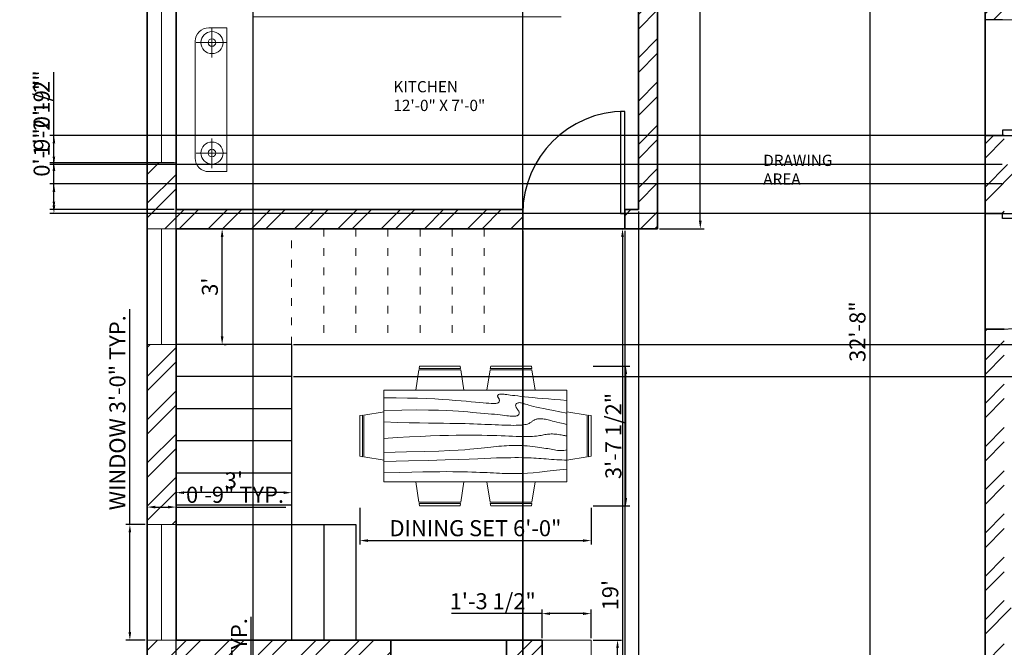
# Model space of a CAD drawing. Units: inches. Extents: x 28986 to 29505, y -162 to 451.
# Tile 3 of 6: x 29011 to 29318, y 32 to 228. Entities that reach past the tile are written whole.
import ezdxf

# ---------------------------------------------------------------- set-up
doc = ezdxf.new("R2010")
doc.units = ezdxf.units.IN
doc.linetypes.add('ACAD_ISO03W100', pattern=[30, 12, -18])
doc.layers.get('Defpoints').update_dxf_attribs({"color": 120})
for name, color, linetype, lineweight, true_color in [('A-ANNO-DIMS', 9, 'Continuous', 18, 0xafd9aa), ('A-FLOR-CASE', 32, 'Continuous', 18, 0xcd6928), ('A-FLOR-STRS', 32, 'Continuous', 25, 0xcd6928), ('A-FLOR-STRS-OVHD', 32, 'ACAD_ISO03W100', 18, 0xcd6928)]:
    doc.layers.add(name, color=color, linetype=linetype, lineweight=lineweight, true_color=true_color)
for name, color, linetype, lineweight in [('A-AREA-IDEN', 6, 'Continuous', 18), ('A-EQPM', 8, 'Continuous', 18), ('A-GLAZ', 4, 'Continuous', 18), ('A-WALL', 7, 'Continuous', 35), ('A-WALL-PATT', 1, 'Continuous', 13), ('DOOR', 2, 'Continuous', 25), ('FURNITURE', 241, 'Continuous', 18)]:
    doc.layers.add(name, color=color, linetype=linetype, lineweight=lineweight)
doc.styles.get("Standard").update_dxf_attribs({"font": 'arial.ttf'})
doc.dimstyles.new('ISO-25', dxfattribs={"dimtxt": 5, "dimasz": 2.5, "dimexe": 1.25, "dimexo": 0.625, "dimtad": 1, "dimdec": 0, "dimlunit": 3, "dimtxsty": 'Standard', "dimcen": 2.5, "dimadec": 0, "dimazin": 0, "dimtfac": 1, "dimtdec": 0, "dimtmove": 0, "dimatfit": 3, "dimfxl": 1, "dimarcsym": 0})

# ---------------------------------------------------------------- blocks, each defined once
blk = doc.blocks.new('*D1')
at = {"layer": 'A-ANNO-DIMS', "color": 0, "lineweight": -2, "transparency": 16777216}
for p, q in [((29075.13, 162.7), (29075.76, 162.7)), ((29074.51, 129.2), (29074.51, 160.2)), ((29075.13, 126.7), (29075.76, 126.7))]:
    blk.add_line(p, q, dxfattribs=at)
at = {"layer": 'A-ANNO-DIMS', "color": 0, "transparency": 16777216}
for points in [[(29074.09, 160.2), (29074.92, 160.2), (29074.51, 162.7)], [(29074.09, 129.2), (29074.92, 129.2), (29074.51, 126.7)]]:
    blk.add_solid(points, dxfattribs=at)
at = {"layer": 'Defpoints', "color": 0, "transparency": 16777216}
for p in [(29074.51, 162.7), (29074.51, 162.7), (29074.51, 126.7)]:
    blk.add_point(p, dxfattribs=at)
at = {"layer": 'A-ANNO-DIMS', "color": 0, "transparency": 16777216, "insert": (29071.33, 144.7), "char_height": 5, "attachment_point": 5, "rotation": 90}
blk.add_mtext("3'", dxfattribs=at)
blk = doc.blocks.new('*D2')
at = {"layer": 'A-ANNO-DIMS', "color": 0, "lineweight": -2, "transparency": 16777216}
for p, q in [((29060.16, 80.07), (29060.16, 79.34)), ((29093.66, 80.59), (29062.66, 80.59)), ((29096.16, 80.07), (29096.16, 79.34))]:
    blk.add_line(p, q, dxfattribs=at)
at = {"layer": 'A-ANNO-DIMS', "color": 0, "transparency": 16777216}
for points in [[(29062.66, 81), (29062.66, 80.17), (29060.16, 80.59)], [(29093.66, 81), (29093.66, 80.17), (29096.16, 80.59)]]:
    blk.add_solid(points, dxfattribs=at)
at = {"layer": 'Defpoints', "color": 0, "transparency": 16777216}
for p in [(29060.16, 80.7), (29060.16, 80.59), (29096.16, 80.7)]:
    blk.add_point(p, dxfattribs=at)
at = {"layer": 'A-ANNO-DIMS', "color": 0, "transparency": 16777216, "insert": (29078.16, 83.77), "char_height": 5, "attachment_point": 5}
blk.add_mtext("3'", dxfattribs=at)
blk = doc.blocks.new('*U5')
for p, q in [((0, 0), (0, -6)), ((-40, 0), (-40, -6))]:
    blk.add_line(p, q)
blk.add_lwpolyline([(0, 0), (0, 40), (-1.75, 40), (-1.75, 0)], close=True)
blk.add_arc((0, 0), 40, 90, 180)
blk = doc.blocks.new('*U7')
for p, q in [((-40, 0), (-40, 6)), ((0, 0), (0, 6))]:
    blk.add_line(p, q)
blk.add_lwpolyline([(0, 0), (0, -40), (-1.75, -40), (-1.75, 0)], close=True)
blk.add_arc((0, 0), 40, 180, 270)
blk = doc.blocks.new('*U8')
for p, q in [((0, 0), (0, 6)), ((40, 0), (40, 6))]:
    blk.add_line(p, q)
blk.add_lwpolyline([(0, 0), (0, -40), (1.75, -40), (1.75, 0)], close=True)
blk.add_arc((0, 0), 40, 270, 0)
blk = doc.blocks.new('tv')
for p, q in [((18.34, 53.39), (15.62, 57.31)), ((15.62, 57.31), (15.62, 11.74)), ((15.62, 11.74), (18.34, 14.53))]:
    blk.add_line(p, q)
blk.add_lwpolyline([(18.34, 0), (0, 0), (0, 65.9), (18.34, 65.9)], close=True)
blk = doc.blocks.new('Dining Set - 36 x 72 in.')
for p, q in [((-22, 27.5), (-22.1562, 26.50042)), ((-22, 27.5), (-6, 27.5)), ((-5.8437, 26.49966), (-6, 27.5)), ((6, 27.5), (5.8438, 26.50042)), ((6, 27.5), (22, 27.5)), ((22.1563, 26.49966), (22, 27.5)), ((-22.2343, 26.00059), (-23.4847, 17.99762)), ((-22.2304, 26), (-5.7608, 26)), ((-5.8416, 26.5), (-22.1534, 26.5)), ((-4.5152, 17.99762), (-5.7655, 25.99926)), ((5.7657, 26.00059), (4.5153, 17.99762)), ((5.7696, 26), (22.2392, 26)), ((22.1584, 26.5), (5.8466, 26.5)), ((23.4848, 17.99762), (22.2345, 25.99926)), ((36, 18), (-36, 18)), ((-36, 18), (-36, -18)), ((36, -18), (36, 18)), ((-45.5, 8), (-44.5004, 8.15617)), ((-45.5, 8), (-45.5, -8)), ((-44.5, -8.15843), (-44.5, 8.15338)), ((-44.0006, 8.23428), (-35.9976, 9.48474)), ((-44, 8.23041), (-44, -8.23915)), ((44.0006, 8.23428), (35.9976, 9.48474)), ((44, 8.23041), (44, -8.23915)), ((44.5, -8.15843), (44.5, 8.15338)), ((45.5, 8), (44.5005, 8.15617)), ((45.5, 8), (45.5, -8)), ((-44.4997, -8.15631), (-45.5, -8)), ((-35.9976, -9.48476), (-43.9993, -8.2345)), ((35.9976, -9.48476), (43.9993, -8.2345)), ((44.4997, -8.15631), (45.5, -8)), ((-36, -18), (36, -18)), ((-22.2343, -26.0006), (-23.4847, -17.99762)), ((-4.5152, -17.99762), (-5.7655, -25.99928)), ((5.7657, -26.0006), (4.5153, -17.99762)), ((23.4848, -17.99762), (22.2345, -25.99928)), ((-22.2304, -26), (-5.7608, -26)), ((-22, -27.5), (-22.1562, -26.50044)), ((-5.8416, -26.5), (-22.1534, -26.5)), ((-5.8437, -26.49967), (-6, -27.5)), ((5.7696, -26), (22.2392, -26)), ((6, -27.5), (5.8438, -26.50044)), ((22.1584, -26.5), (5.8466, -26.5)), ((22.1563, -26.49967), (22, -27.5)), ((-22, -27.5), (-6, -27.5)), ((6, -27.5), (22, -27.5))]:
    blk.add_line(p, q)
for points in [[(-36, 15), (-31.1772, 14.97754), (-26.8079, 14.91406), (-22.8538, 14.81543), (-19.276, 14.6875), (-16.0362, 14.53613), (-13.0957, 14.36718), (-10.4159, 14.18652), (-7.9583, 14), (-5.6904, 13.81315), (-3.6035, 13.63021), (-1.6954, 13.45508), (0.0365, 13.29166), (1.5945, 13.14388), (2.9811, 13.01562), (4.1988, 12.9108), (5.25, 12.83333), (6.1393, 12.78613), (6.8802, 12.76823), (7.4883, 12.77767), (7.9792, 12.8125), (8.3685, 12.87077), (8.6719, 12.95052), (8.9049, 13.0498), (9.0833, 13.16666), (9.2205, 13.29899), (9.3216, 13.44401), (9.3895, 13.59879), (9.4271, 13.76041), (9.4373, 13.92594), (9.4232, 14.09245), (9.3875, 14.257), (9.3333, 14.41666), (9.2638, 14.56917), (9.1836, 14.71484), (9.0975, 14.85465), (9.0104, 14.98958), (8.9272, 15.1206), (8.8529, 15.2487), (8.7922, 15.37483), (8.75, 15.5), (8.7305, 15.62467), (8.7344, 15.74739), (8.7617, 15.86621), (8.8125, 15.97916), (8.8867, 16.08431), (8.9844, 16.17968), (9.1055, 16.26334), (9.25, 16.33333), (9.4189, 16.38802), (9.6172, 16.42708), (9.8506, 16.45052), (10.125, 16.45833), (10.4463, 16.45052), (10.8203, 16.42708), (11.2529, 16.38802), (11.75, 16.33333), (12.3184, 16.26318), (12.9694, 16.17838), (13.7151, 16.07991), (14.5677, 15.96875), (15.5395, 15.84586), (16.6426, 15.71224), (17.8893, 15.56884), (19.2917, 15.41666), (20.859, 15.25667), (22.5879, 15.08984), (24.4721, 14.91715), (26.5052, 14.73958), (28.6809, 14.5581), (30.9929, 14.3737), (33.4347, 14.18733), (36, 14)], [(-36, 10), (-28.9766, 10.14274), (-23.1725, 10.20442), (-18.4241, 10.19775), (-14.5677, 10.13541), (-11.4399, 10.03011), (-8.877, 9.89453), (-6.7154, 9.74137), (-4.7917, 9.58333), (-2.9698, 9.43082), (-1.2246, 9.28515), (0.4415, 9.14534), (2.026, 9.01041), (3.5266, 8.87939), (4.9408, 8.7513), (6.266, 8.62516), (7.5, 8.5), (8.6411, 8.37549), (9.6914, 8.2539), (10.6538, 8.13818), (11.5312, 8.03125), (12.3267, 7.93603), (13.043, 7.85547), (13.6831, 7.79248), (14.25, 7.75), (14.7471, 7.7303), (15.1797, 7.73307), (15.5537, 7.75732), (15.875, 7.80208), (16.1494, 7.86637), (16.3828, 7.94922), (16.5811, 8.04964), (16.75, 8.16666), (16.8944, 8.29915), (17.0143, 8.44531), (17.1089, 8.60319), (17.1771, 8.77083), (17.218, 8.94629), (17.2305, 9.1276), (17.2137, 9.31282), (17.1667, 9.5), (17.0895, 9.6875), (16.987, 9.875), (16.8649, 10.0625), (16.7292, 10.25), (16.5856, 10.4375), (16.4401, 10.625), (16.2985, 10.8125), (16.1667, 11), (16.05, 11.18733), (15.9518, 11.3737), (15.8752, 11.5581), (15.8229, 11.73958), (15.798, 11.91715), (15.8034, 12.08984), (15.842, 12.25667), (15.9167, 12.41666), (16.0295, 12.56836), (16.1784, 12.70833), (16.3605, 12.83268), (16.5729, 12.9375), (16.8127, 13.01888), (17.0768, 13.07291), (17.3625, 13.0957), (17.6667, 13.08333), (17.9894, 13.03312), (18.3418, 12.94726), (18.7382, 12.82918), (19.1927, 12.68229), (19.7195, 12.51001), (20.3327, 12.31575), (21.0465, 12.10294), (21.875, 11.875), (22.8357, 11.63354), (23.959, 11.37304), (25.2786, 11.08618), (26.8282, 10.76562), (28.6414, 10.40405), (30.752, 9.99414), (33.1936, 9.52856), (36, 9)], [(-36, 5.5), (-30.7157, 5.3348), (-26.069, 5.20963), (-21.9946, 5.11767), (-18.4271, 5.05208), (-15.3009, 5.00602), (-12.5508, 4.97265), (-10.1112, 4.94515), (-7.9167, 4.91666), (-5.909, 4.88167), (-4.0586, 4.83984), (-2.3429, 4.79215), (-0.7396, 4.73958), (0.7739, 4.6831), (2.22, 4.6237), (3.6213, 4.56233), (5, 4.5), (6.373, 4.43782), (7.7344, 4.3776), (9.0723, 4.32129), (10.375, 4.27083), (11.6309, 4.22819), (12.8281, 4.19531), (13.9551, 4.17415), (15, 4.16666), (15.954, 4.17448), (16.819, 4.19791), (17.6001, 4.23698), (18.3021, 4.29166), (18.9299, 4.36198), (19.4883, 4.44791), (19.9823, 4.54948), (20.4167, 4.66666), (20.7969, 4.79899), (21.1302, 4.94401), (21.4245, 5.09879), (21.6875, 5.26041), (21.9271, 5.42594), (22.1511, 5.59245), (22.3672, 5.757), (22.5834, 5.91666), (22.8065, 6.06868), (23.0404, 6.21093), (23.2879, 6.34147), (23.5521, 6.45833), (23.8358, 6.55957), (24.142, 6.64323), (24.4735, 6.70735), (24.8334, 6.75), (25.2235, 6.76969), (25.642, 6.76692), (26.0858, 6.74267), (26.5521, 6.69791), (27.0379, 6.63362), (27.5404, 6.55078), (28.0565, 6.45036), (28.5834, 6.33333), (29.1242, 6.19987), (29.7071, 6.04687), (30.3661, 5.87044), (31.1354, 5.66666), (32.0493, 5.43164), (33.142, 5.16146), (34.4475, 4.85221), (36, 4.5)], [(-36, -1), (-30.7915, -0.6591), (-26.0195, -0.38216), (-21.6519, -0.16284), (-17.6563, 0.00521), (-14.0005, 0.12833), (-10.6523, 0.21289), (-7.5796, 0.26522), (-4.75, 0.29166), (-2.134, 0.29793), (0.2878, 0.28711), (2.5317, 0.26163), (4.6146, 0.22396), (6.5529, 0.17651), (8.3633, 0.12174), (10.0623, 0.06209), (11.6667, 0), (13.1899, -0.06201), (14.6341, -0.1211), (15.9982, -0.17432), (17.2813, -0.21875), (18.4823, -0.25147), (19.6003, -0.26953), (20.6343, -0.27002), (21.5834, -0.25), (22.4481, -0.20768), (23.2357, -0.14584), (23.9549, -0.06836), (24.6146, 0.02083), (25.2235, 0.11784), (25.7904, 0.21875), (26.3241, 0.31966), (26.8334, 0.41666), (27.3265, 0.50618), (27.8099, 0.58593), (28.2894, 0.65397), (28.7709, 0.70833), (29.2601, 0.74707), (29.763, 0.76823), (30.2855, 0.76985), (30.8334, 0.75), (31.4088, 0.70784), (31.9994, 0.64713), (32.589, 0.57275), (33.1615, 0.48958), (33.7008, 0.4025), (34.1908, 0.3164), (34.6153, 0.23616), (34.9584, 0.16666), (35.2099, 0.11165), (35.3848, 0.07031), (35.504, 0.04069), (35.5886, 0.02083), (35.6594, 0.00879), (35.7377, 0.0026), (35.8442, 0.00032), (36, 0)], [(-36, -6.5), (-27.1843, -6.31267), (-20.084, -6.1263), (-14.469, -5.9419), (-10.1094, -5.76042), (-6.7752, -5.58285), (-4.2363, -5.41016), (-2.2629, -5.24333), (-0.625, -5.08334), (0.8708, -4.93099), (2.2715, -4.78646), (3.5872, -4.64974), (4.8281, -4.52084), (6.0046, -4.39974), (7.127, -4.28646), (8.2053, -4.18099), (9.25, -4.08334), (10.2705, -3.99382), (11.2734, -3.91407), (12.2647, -3.84603), (13.25, -3.79167), (14.2354, -3.75293), (15.2266, -3.73177), (16.2295, -3.73015), (17.25, -3.75), (18.2912, -3.79248), (19.3451, -3.85547), (20.4009, -3.93604), (21.4479, -4.03125), (22.4754, -4.13819), (23.4727, -4.25391), (24.4289, -4.37549), (25.3334, -4.5), (26.1785, -4.62492), (26.9694, -4.74935), (27.7145, -4.87281), (28.4219, -4.99479), (29.1, -5.11483), (29.7572, -5.23242), (30.4016, -5.34709), (31.0417, -5.45834), (31.6837, -5.56437), (32.3262, -5.65821), (32.9658, -5.73153), (33.599, -5.77604), (34.2224, -5.78345), (34.8327, -5.74545), (35.4264, -5.65373), (36, -5.5)], [(-36, -10), (-26.4022, -9.81299), (-18.4675, -9.62891), (-11.9839, -9.45069), (-6.7396, -9.28125), (-2.5226, -9.12354), (0.8789, -8.98047), (3.6769, -8.85498), (6.0833, -8.75), (8.2767, -8.66765), (10.3021, -8.60677), (12.1712, -8.56543), (13.8958, -8.54167), (15.4876, -8.53353), (16.9583, -8.53907), (18.3197, -8.55632), (19.5834, -8.58334), (20.7616, -8.61841), (21.8685, -8.66081), (22.9188, -8.71004), (23.9271, -8.76563), (24.9081, -8.82707), (25.8763, -8.89388), (26.8465, -8.96558), (27.8334, -9.04167), (28.8474, -9.12118), (29.8828, -9.20117), (30.93, -9.27824), (31.9792, -9.34896), (33.0205, -9.40991), (34.0443, -9.45768), (35.0407, -9.48885), (36, -9.5)], [(-36, -14.5), (-30.0881, -14.33513), (-25.0332, -14.21224), (-20.7312, -14.12647), (-17.0781, -14.07292), (-13.97, -14.04671), (-11.3027, -14.04297), (-8.9724, -14.05681), (-6.875, -14.08334), (-4.9224, -14.11833), (-3.0905, -14.16016), (-1.3709, -14.20785), (0.2448, -14.26042), (1.7647, -14.3169), (3.1973, -14.3763), (4.5507, -14.43767), (5.8333, -14.5), (7.0554, -14.5621), (8.235, -14.62175), (9.3922, -14.67652), (10.5469, -14.72396), (11.7192, -14.76164), (12.929, -14.78711), (14.1965, -14.79794), (15.5417, -14.79167), (16.9933, -14.76424), (18.6152, -14.70508), (20.4804, -14.60197), (22.6615, -14.44271), (25.2312, -14.21509), (28.2624, -13.9069), (31.8277, -13.50594), (36, -13)]]:
    blk.add_lwpolyline(points)
blk = doc.blocks.new('STOVE')
for p, q in [((-46.84, 5.62), (-46.82, 11.55)), ((-5.51, 5.62), (-5.49, 11.55)), ((-46.84, 5.62), (-52.42, 5.62)), ((-46.84, 5.62), (-46.84, 0.29)), ((-46.84, 5.62), (-41.4, 5.62)), ((-5.51, 5.62), (-11.1, 5.62)), ((-5.51, 5.62), (-5.51, 0.29)), ((-5.51, 5.62), (-0.08, 5.62))]:
    blk.add_line(p, q)
blk.add_lwpolyline([(-48.78, 11.85), (-5, 11.85, -0.414214), (0, 6.85), (0, 0), (-53.78, 0), (-53.78, 6.85, -0.414214)], format="xyb", close=True)
for centre, radius in [((-46.84, 5.62), 4.14), ((-5.51, 5.62), 4.14), ((-46.84, 5.62), 1.41), ((-5.51, 5.62), 1.41)]:
    blk.add_circle(centre, radius)
blk = doc.blocks.new('*D18')
at = {"layer": 'A-ANNO-DIMS', "color": 0, "lineweight": -2, "transparency": 16777216}
for p, q in [((29278.83, 326.7), (29274.99, 326.7)), ((29276.24, 324.2), (29276.24, -62.8)), ((29278.83, -65.3), (29274.99, -65.3))]:
    blk.add_line(p, q, dxfattribs=at)
at = {"layer": 'A-ANNO-DIMS', "color": 0, "transparency": 16777216}
for points in [[(29275.82, 324.2), (29276.65, 324.2), (29276.24, 326.7)], [(29275.82, -62.8), (29276.65, -62.8), (29276.24, -65.3)]]:
    blk.add_solid(points, dxfattribs=at)
at = {"layer": 'Defpoints', "color": 0, "transparency": 16777216}
for p in [(29279.46, 326.7), (29276.24, -65.3), (29279.46, -65.3)]:
    blk.add_point(p, dxfattribs=at)
at = {"layer": 'A-ANNO-DIMS', "color": 0, "transparency": 16777216, "insert": (29273.06, 130.7), "char_height": 5, "attachment_point": 5, "rotation": 90}
blk.add_mtext('32\'-8"', dxfattribs=at)
blk = doc.blocks.new('*D19')
at = {"layer": 'A-ANNO-DIMS', "color": 0, "lineweight": -2, "transparency": 16777216}
for p, q in [((29196.21, 162.7), (29200.48, 162.7)), ((29199.23, 160.2), (29199.23, -62.8)), ((29196.21, -65.3), (29200.48, -65.3))]:
    blk.add_line(p, q, dxfattribs=at)
at = {"layer": 'A-ANNO-DIMS', "color": 0, "transparency": 16777216}
for points in [[(29198.82, 160.2), (29199.65, 160.2), (29199.23, 162.7)], [(29198.82, -62.8), (29199.65, -62.8), (29199.23, -65.3)]]:
    blk.add_solid(points, dxfattribs=at)
at = {"layer": 'Defpoints', "color": 0, "transparency": 16777216}
for p in [(29195.59, 162.7), (29195.59, -65.3), (29199.23, -65.3)]:
    blk.add_point(p, dxfattribs=at)
at = {"layer": 'A-ANNO-DIMS', "color": 0, "transparency": 16777216, "insert": (29196.05, 48.7), "char_height": 5, "attachment_point": 5, "rotation": 90}
blk.add_mtext("19'", dxfattribs=at)
blk = doc.blocks.new('*D22')
at = {"layer": 'A-ANNO-DIMS', "color": 0, "lineweight": -2, "transparency": 16777216}
for p, q in [((29210.78, 326.7), (29224.71, 326.7)), ((29223.46, 165.2), (29223.46, 324.2)), ((29210.78, 162.7), (29224.71, 162.7))]:
    blk.add_line(p, q, dxfattribs=at)
at = {"layer": 'A-ANNO-DIMS', "color": 0, "transparency": 16777216}
for points in [[(29223.04, 324.2), (29223.87, 324.2), (29223.46, 326.7)], [(29223.04, 165.2), (29223.87, 165.2), (29223.46, 162.7)]]:
    blk.add_solid(points, dxfattribs=at)
at = {"layer": 'Defpoints', "color": 0, "transparency": 16777216}
for p in [(29210.16, 326.7), (29223.46, 326.7), (29210.16, 162.7)]:
    blk.add_point(p, dxfattribs=at)
at = {"layer": 'A-ANNO-DIMS', "color": 0, "transparency": 16777216, "insert": (29220.28, 244.7), "char_height": 5, "attachment_point": 5, "rotation": 90}
blk.add_mtext('13\'-8"', dxfattribs=at)
blk = doc.blocks.new('WIN-48IN')
for p, q in [((9, 48), (0, 48)), ((4.5, 0), (4.5, 48)), ((9, 0), (0, 0))]:
    blk.add_line(p, q)
blk = doc.blocks.new('WIN-36IN')
for p, q in [((9, 36), (0, 36)), ((4.5, 0), (4.5, 36)), ((9, 0), (0, 0))]:
    blk.add_line(p, q)
blk = doc.blocks.new('*D41')
at = {"layer": 'A-ANNO-DIMS', "color": 0, "lineweight": -2, "transparency": 16777216}
for p, q in [((29045.76, 70.7), (29045.76, 137.72)), ((29050.53, 70.7), (29044.51, 70.7)), ((29045.76, 37.2), (29045.76, 68.2)), ((29050.53, 34.7), (29044.51, 34.7))]:
    blk.add_line(p, q, dxfattribs=at)
at = {"layer": 'A-ANNO-DIMS', "color": 0, "transparency": 16777216}
for points in [[(29045.34, 68.2), (29046.17, 68.2), (29045.76, 70.7)], [(29045.34, 37.2), (29046.17, 37.2), (29045.76, 34.7)]]:
    blk.add_solid(points, dxfattribs=at)
at = {"layer": 'Defpoints', "color": 0, "transparency": 16777216}
for p in [(29045.76, 70.7), (29051.16, 70.7), (29051.16, 34.7)]:
    blk.add_point(p, dxfattribs=at)
at = {"layer": 'A-ANNO-DIMS', "color": 0, "transparency": 16777216, "insert": (29042.54, 105.46), "char_height": 5, "attachment_point": 5, "rotation": 90}
blk.add_mtext('WINDOW 3\'-0" TYP.', dxfattribs=at)
blk = doc.blocks.new('*D42')
at = {"layer": 'A-ANNO-DIMS', "color": 0, "lineweight": -2, "transparency": 16777216}
for p, q in [((29051.16, 71.32), (29051.16, 77.35)), ((29060.16, 71.32), (29060.16, 77.35)), ((29053.66, 76.1), (29057.66, 76.1)), ((29060.16, 76.1), (29094.38, 76.1))]:
    blk.add_line(p, q, dxfattribs=at)
at = {"layer": 'A-ANNO-DIMS', "color": 0, "transparency": 16777216}
for points in [[(29053.66, 76.52), (29053.66, 75.68), (29051.16, 76.1)], [(29057.66, 76.52), (29057.66, 75.68), (29060.16, 76.1)]]:
    blk.add_solid(points, dxfattribs=at)
at = {"layer": 'Defpoints', "color": 0, "transparency": 16777216}
for p in [(29060.16, 76.1), (29051.16, 70.7), (29060.16, 70.7)]:
    blk.add_point(p, dxfattribs=at)
at = {"layer": 'A-ANNO-DIMS', "color": 0, "transparency": 16777216, "insert": (29078.52, 79.28), "char_height": 5, "attachment_point": 5}
blk.add_mtext('0\'-9" TYP.', dxfattribs=at)
blk = doc.blocks.new('*D52')
at = {"layer": 'A-ANNO-DIMS', "color": 0, "lineweight": -2, "transparency": 16777216}
for p, q in [((29083.58, 8.15), (29083.58, 41.9)), ((29081.15, 8.15), (29084.83, 8.15)), ((29083.58, -7.58), (29083.58, 5.65)), ((29081.15, -10.08), (29084.83, -10.08))]:
    blk.add_line(p, q, dxfattribs=at)
at = {"layer": 'A-ANNO-DIMS', "color": 0, "transparency": 16777216}
for points in [[(29083.17, 5.65), (29084, 5.65), (29083.58, 8.15)], [(29083.17, -7.58), (29084, -7.58), (29083.58, -10.08)]]:
    blk.add_solid(points, dxfattribs=at)
at = {"layer": 'Defpoints', "color": 0, "transparency": 16777216}
for p in [(29080.53, 8.15), (29083.58, 8.15), (29080.53, -10.08)]:
    blk.add_point(p, dxfattribs=at)
at = {"layer": 'A-ANNO-DIMS', "color": 0, "transparency": 16777216, "insert": (29080.4, 26.28), "char_height": 5, "attachment_point": 5, "rotation": 90}
blk.add_mtext('1\'-6" TYP.', dxfattribs=at)
blk = doc.blocks.new('*D55')
at = {"layer": 'A-ANNO-DIMS', "color": 0, "lineweight": -2, "transparency": 16777216}
for p, q in [((29190.06, 34.7), (29198.93, 34.7)), ((29197.68, -17.72), (29197.68, 32.2)), ((29190.06, -20.22), (29198.93, -20.22))]:
    blk.add_line(p, q, dxfattribs=at)
at = {"layer": 'A-ANNO-DIMS', "color": 0, "transparency": 16777216}
for points in [[(29197.26, 32.2), (29198.09, 32.2), (29197.68, 34.7)], [(29197.26, -17.72), (29198.09, -17.72), (29197.68, -20.22)]]:
    blk.add_solid(points, dxfattribs=at)
at = {"layer": 'Defpoints', "color": 0, "transparency": 16777216}
for p in [(29189.44, 34.7), (29197.68, 34.7), (29189.44, -20.22)]:
    blk.add_point(p, dxfattribs=at)
at = {"layer": 'A-ANNO-DIMS', "color": 0, "transparency": 16777216, "insert": (29194.55, 7.24), "char_height": 5, "attachment_point": 5, "rotation": 90}
blk.add_mtext('TV 4\'-7"', dxfattribs=at)
blk = doc.blocks.new('*D56')
at = {"layer": 'A-ANNO-DIMS', "color": 0, "lineweight": -2, "transparency": 16777216}
for p, q in [((29174.16, 35.32), (29174.16, 44.19)), ((29189.44, 35.32), (29189.44, 44.19)), ((29174.16, 42.94), (29145.94, 42.94)), ((29186.94, 42.94), (29176.66, 42.94))]:
    blk.add_line(p, q, dxfattribs=at)
at = {"layer": 'A-ANNO-DIMS', "color": 0, "transparency": 16777216}
for points in [[(29176.66, 43.35), (29176.66, 42.52), (29174.16, 42.94)], [(29186.94, 43.35), (29186.94, 42.52), (29189.44, 42.94)]]:
    blk.add_solid(points, dxfattribs=at)
at = {"layer": 'Defpoints', "color": 0, "transparency": 16777216}
for p in [(29174.16, 42.94), (29174.16, 34.7), (29189.44, 34.7)]:
    blk.add_point(p, dxfattribs=at)
at = {"layer": 'A-ANNO-DIMS', "color": 0, "transparency": 16777216, "insert": (29158.8, 46.15), "char_height": 5, "attachment_point": 5}
blk.add_mtext('1\'-3 1/2"', dxfattribs=at)
blk = doc.blocks.new('*D61')
at = {"layer": 'A-ANNO-DIMS', "color": 0, "lineweight": -2, "transparency": 16777216}
for p, q in [((29117.41, 75.85), (29117.41, 64.42)), ((29189.44, 75.85), (29189.44, 64.42)), ((29119.91, 65.67), (29186.94, 65.67))]:
    blk.add_line(p, q, dxfattribs=at)
at = {"layer": 'A-ANNO-DIMS', "color": 0, "transparency": 16777216}
for points in [[(29119.91, 66.08), (29119.91, 65.25), (29117.41, 65.67)], [(29186.94, 66.08), (29186.94, 65.25), (29189.44, 65.67)]]:
    blk.add_solid(points, dxfattribs=at)
at = {"layer": 'Defpoints', "color": 0, "transparency": 16777216}
for p in [(29117.41, 76.47), (29189.44, 76.47), (29189.44, 65.67)]:
    blk.add_point(p, dxfattribs=at)
at = {"layer": 'A-ANNO-DIMS', "color": 0, "transparency": 16777216, "insert": (29153.42, 68.88), "char_height": 5, "attachment_point": 5}
blk.add_mtext('DINING SET 6\'-0"', dxfattribs=at)
blk = doc.blocks.new('*D62')
at = {"layer": 'A-ANNO-DIMS', "color": 0, "lineweight": -2, "transparency": 16777216}
for p, q in [((29190.06, 120), (29201.49, 120)), ((29200.24, 78.97), (29200.24, 117.5)), ((29190.06, 76.47), (29201.49, 76.47))]:
    blk.add_line(p, q, dxfattribs=at)
at = {"layer": 'A-ANNO-DIMS', "color": 0, "transparency": 16777216}
for points in [[(29199.82, 117.5), (29200.66, 117.5), (29200.24, 120)], [(29199.82, 78.97), (29200.66, 78.97), (29200.24, 76.47)]]:
    blk.add_solid(points, dxfattribs=at)
at = {"layer": 'Defpoints', "color": 0, "transparency": 16777216}
for p in [(29189.44, 120), (29200.24, 120), (29189.44, 76.47)]:
    blk.add_point(p, dxfattribs=at)
at = {"layer": 'A-ANNO-DIMS', "color": 0, "transparency": 16777216, "insert": (29197.03, 98.24), "char_height": 5, "attachment_point": 5, "rotation": 90}
blk.add_mtext('3\'-7 1/2"', dxfattribs=at)
blk = doc.blocks.new('*D64')
at = {"layer": 'A-ANNO-DIMS', "color": 0, "lineweight": -2, "transparency": 16777216}
for p, q in [((29060.16, 26.32), (29060.16, 442)), ((29168.16, 26.32), (29168.16, 442)), ((29165.66, 440.75), (29062.66, 440.75))]:
    blk.add_line(p, q, dxfattribs=at)
at = {"layer": 'A-ANNO-DIMS', "color": 0, "transparency": 16777216}
for points in [[(29062.66, 441.17), (29062.66, 440.33), (29060.16, 440.75)], [(29165.66, 441.17), (29165.66, 440.33), (29168.16, 440.75)]]:
    blk.add_solid(points, dxfattribs=at)
at = {"layer": 'Defpoints', "color": 0, "transparency": 16777216}
for p in [(29060.16, 440.75), (29060.16, 25.7), (29168.16, 25.7)]:
    blk.add_point(p, dxfattribs=at)
at = {"layer": 'A-ANNO-DIMS', "color": 0, "transparency": 16777216, "insert": (29114.16, 443.93), "char_height": 5, "attachment_point": 5}
blk.add_mtext('9\'-0"', dxfattribs=at)
blk = doc.blocks.new('*D71')
at = {"layer": 'A-ANNO-DIMS', "color": 0, "lineweight": -2, "transparency": 16777216}
for p, q in [((29022.11, 183.24), (29022.11, 211.46)), ((29059.53, 183.24), (29020.86, 183.24)), ((29022.11, 171.2), (29022.11, 180.74)), ((29059.53, 168.7), (29020.86, 168.7))]:
    blk.add_line(p, q, dxfattribs=at)
at = {"layer": 'A-ANNO-DIMS', "color": 0, "transparency": 16777216}
for points in [[(29021.69, 180.74), (29022.52, 180.74), (29022.11, 183.24)], [(29021.69, 171.2), (29022.52, 171.2), (29022.11, 168.7)]]:
    blk.add_solid(points, dxfattribs=at)
at = {"layer": 'Defpoints', "color": 0, "transparency": 16777216}
for p in [(29022.11, 183.24), (29060.16, 183.24), (29060.16, 168.7)]:
    blk.add_point(p, dxfattribs=at)
at = {"layer": 'A-ANNO-DIMS', "color": 0, "transparency": 16777216, "insert": (29018.9, 198.6), "char_height": 5, "attachment_point": 5, "rotation": 90}
blk.add_mtext('1\'-2 1/2"', dxfattribs=at)
blk = doc.blocks.new('*D84')
at = {"layer": 'A-ANNO-DIMS', "color": 0, "lineweight": -2, "transparency": 16777216}
for p, q in [((29168.16, 162.07), (29168.16, -158.6)), ((29199.96, 162.07), (29199.96, -158.6)), ((29170.66, -157.35), (29197.46, -157.35))]:
    blk.add_line(p, q, dxfattribs=at)
at = {"layer": 'A-ANNO-DIMS', "color": 0, "transparency": 16777216}
for points in [[(29170.66, -156.93), (29170.66, -157.77), (29168.16, -157.35)], [(29197.46, -156.93), (29197.46, -157.77), (29199.96, -157.35)]]:
    blk.add_solid(points, dxfattribs=at)
at = {"layer": 'Defpoints', "color": 0, "transparency": 16777216}
for p in [(29168.16, 162.7), (29199.96, 162.7), (29199.96, -157.35)]:
    blk.add_point(p, dxfattribs=at)
at = {"layer": 'A-ANNO-DIMS', "color": 0, "transparency": 16777216, "insert": (29184.06, -154.17), "char_height": 5, "attachment_point": 5}
blk.add_mtext('2\'-8"', dxfattribs=at)
blk = doc.blocks.new('*D86')
at = {"layer": 'A-ANNO-DIMS', "color": 0, "lineweight": -2, "transparency": 16777216}
for p, q in [((29022.11, 176.7), (29022.11, 193.74)), ((29317.53, 176.7), (29020.86, 176.7)), ((29022.11, 169.99), (29022.11, 174.2)), ((29317.53, 167.49), (29020.86, 167.49))]:
    blk.add_line(p, q, dxfattribs=at)
at = {"layer": 'A-ANNO-DIMS', "color": 0, "transparency": 16777216}
for points in [[(29021.69, 174.2), (29022.52, 174.2), (29022.11, 176.7)], [(29021.69, 169.99), (29022.52, 169.99), (29022.11, 167.49)]]:
    blk.add_solid(points, dxfattribs=at)
at = {"layer": 'Defpoints', "color": 0, "transparency": 16777216}
for p in [(29022.11, 176.7), (29318.16, 176.7), (29318.16, 167.49)]:
    blk.add_point(p, dxfattribs=at)
at = {"layer": 'A-ANNO-DIMS', "color": 0, "transparency": 16777216, "insert": (29018.93, 186.47), "char_height": 5, "attachment_point": 5, "rotation": 90}
blk.add_mtext('0\'-9"', dxfattribs=at)
blk = doc.blocks.new('*D87')
at = {"layer": 'A-ANNO-DIMS', "color": 0, "lineweight": -2, "transparency": 16777216}
for p, q in [((29022.11, 191.79), (29022.11, 208.83)), ((29317.53, 191.79), (29020.86, 191.79)), ((29022.11, 185.2), (29022.11, 189.29)), ((29317.53, 182.7), (29020.86, 182.7))]:
    blk.add_line(p, q, dxfattribs=at)
at = {"layer": 'A-ANNO-DIMS', "color": 0, "transparency": 16777216}
for points in [[(29021.69, 189.29), (29022.52, 189.29), (29022.11, 191.79)], [(29021.69, 185.2), (29022.52, 185.2), (29022.11, 182.7)]]:
    blk.add_solid(points, dxfattribs=at)
at = {"layer": 'Defpoints', "color": 0, "transparency": 16777216}
for p in [(29022.11, 191.79), (29318.16, 191.79), (29318.16, 182.7)]:
    blk.add_point(p, dxfattribs=at)
at = {"layer": 'A-ANNO-DIMS', "color": 0, "transparency": 16777216, "insert": (29018.93, 201.56), "char_height": 5, "attachment_point": 5, "rotation": 90}
blk.add_mtext('0\'-9"', dxfattribs=at)
blk = doc.blocks.new('*D88')
at = {"layer": 'A-ANNO-DIMS', "color": 0, "lineweight": -2, "transparency": 16777216}
for p, q in [((29060.16, -16.69), (29060.16, 442)), ((29084.16, -16.69), (29084.16, 442)), ((29062.66, 440.75), (29081.66, 440.75))]:
    blk.add_line(p, q, dxfattribs=at)
at = {"layer": 'A-ANNO-DIMS', "color": 0, "transparency": 16777216}
for points in [[(29062.66, 441.17), (29062.66, 440.33), (29060.16, 440.75)], [(29081.66, 441.17), (29081.66, 440.33), (29084.16, 440.75)]]:
    blk.add_solid(points, dxfattribs=at)
at = {"layer": 'Defpoints', "color": 0, "transparency": 16777216}
for p in [(29084.16, 440.75), (29060.16, -17.32), (29084.16, -17.32)]:
    blk.add_point(p, dxfattribs=at)
at = {"layer": 'A-ANNO-DIMS', "color": 0, "transparency": 16777216, "insert": (29072.16, 443.93), "char_height": 5, "attachment_point": 5}
blk.add_mtext('2\'-0"', dxfattribs=at)
blk = doc.blocks.new('*D91')
at = {"layer": 'A-ANNO-DIMS', "color": 0, "lineweight": -2, "transparency": 16777216}
for p, q in [((29096.78, 126.7), (29501.46, 126.7)), ((29500.21, 124.2), (29500.21, 119.2)), ((29096.78, 116.7), (29501.46, 116.7)), ((29500.21, 116.7), (29500.21, 95.77))]:
    blk.add_line(p, q, dxfattribs=at)
at = {"layer": 'A-ANNO-DIMS', "color": 0, "transparency": 16777216}
for points in [[(29499.79, 124.2), (29500.62, 124.2), (29500.21, 126.7)], [(29499.79, 119.2), (29500.62, 119.2), (29500.21, 116.7)]]:
    blk.add_solid(points, dxfattribs=at)
at = {"layer": 'Defpoints', "color": 0, "transparency": 16777216}
for p in [(29096.16, 126.7), (29096.16, 116.7), (29500.21, 116.7)]:
    blk.add_point(p, dxfattribs=at)
at = {"layer": 'A-ANNO-DIMS', "color": 0, "transparency": 16777216, "insert": (29497.03, 104.99), "char_height": 5, "attachment_point": 5, "rotation": 90}
blk.add_mtext('0\'-10"', dxfattribs=at)
blk = doc.blocks.new('*D98')
at = {"layer": 'A-ANNO-DIMS', "color": 0, "lineweight": -2, "transparency": 16777216}
for p, q in [((29204.16, 168.07), (29204.16, -158.6)), ((29199.96, 162.07), (29199.96, -158.6)), ((29197.46, -157.35), (29194.96, -157.35)), ((29199.96, -157.35), (29204.16, -157.35)), ((29206.66, -157.35), (29223.7, -157.35))]:
    blk.add_line(p, q, dxfattribs=at)
at = {"layer": 'A-ANNO-DIMS', "color": 0, "transparency": 16777216}
for points in [[(29197.46, -156.93), (29197.46, -157.77), (29199.96, -157.35)], [(29206.66, -156.93), (29206.66, -157.77), (29204.16, -157.35)]]:
    blk.add_solid(points, dxfattribs=at)
at = {"layer": 'Defpoints', "color": 0, "transparency": 16777216}
for p in [(29204.16, 168.7), (29199.96, 162.7), (29204.16, -157.35)]:
    blk.add_point(p, dxfattribs=at)
at = {"layer": 'A-ANNO-DIMS', "color": 0, "transparency": 16777216, "insert": (29216.43, -154.17), "char_height": 5, "attachment_point": 5}
blk.add_mtext('0\'-4"', dxfattribs=at)

msp = doc.modelspace()

# ---------------------------------------------------------------- hatches: boundary and pattern name
at = {"layer": 'A-WALL-PATT'}
h = msp.add_hatch(dxfattribs=at)
h.set_pattern_fill('ANSI32', color=256)
h.paths.add_polyline_path([(29174.16, 34.7), (29163.04, 34.7), (29163.04, 29.3), (29163.04, 25.7), (29168.16, 25.7), (29168.16, -119.3), (29174.16, -119.3), (29174.16, -71.3), (29199.96, -71.3), (29199.96, -65.3), (29174.16, -65.3)])
h.paths.add_polyline_path([(29244.8, -65.3), (29235.96, -65.3), (29235.96, -71.3), (29244.8, -71.3)])
h.paths.add_polyline_path([(29318.16, 39.7), (29462.16, 39.7), (29462.16, 44.7), (29318.16, 44.7), (29318.16, 131.49), (29312.16, 131.49), (29312.16, -65.3), (29292.8, -65.3), (29292.8, -71.3), (29312.16, -71.3), (29312.16, -119.3), (29318.16, -119.3)])
h.paths.add_polyline_path([(29219.6, 411.7), (29051.16, 411.7), (29051.16, 368.84), (29060.16, 368.84), (29060.16, 402.7), (29204.16, 402.7), (29219.6, 402.7)])
h.paths.add_polyline_path([(29060.16, 320.84), (29051.16, 320.84), (29051.16, 231.24), (29060.16, 231.24), (29060.16, 252.7)])
h.paths.add_polyline_path([(29210.16, 265.69), (29204.76, 265.69), (29204.16, 265.69), (29204.16, 258.7), (29060.16, 258.7), (29060.16, 252.7), (29204.16, 252.7), (29204.16, 228.7), (29204.16, 168.7), (29199.96, 168.7), (29199.96, 167.47), (29199.96, 162.7), (29210.16, 162.7)])
h.paths.add_polyline_path([(29060.16, 183.24), (29051.16, 183.24), (29051.16, 162.7), (29060.16, 162.7), (29168.16, 162.7), (29168.16, 167.47), (29168.16, 168.7), (29060.16, 168.7)])
h.paths.add_polyline_path([(29060.16, 126.7), (29051.16, 126.7), (29051.16, 70.7), (29060.16, 70.7)])
h.paths.add_polyline_path([(29060.16, 25.7), (29127.04, 25.7), (29127.04, 34.7), (29060.16, 34.7), (29051.16, 34.7), (29051.16, -22.45), (29060.16, -22.45)])
h.paths.add_polyline_path([(29060.16, -70.45), (29051.16, -70.45), (29051.16, -128.3), (29084.16, -128.3), (29084.16, -119.3), (29060.16, -119.3)])
h.paths.add_polyline_path([(29174.16, -119.3), (29168.16, -119.3), (29132.16, -119.3), (29132.16, -128.3), (29174.16, -128.3)])
h.paths.add_polyline_path([(29471.16, 79.78), (29462.16, 79.78), (29462.16, -119.3), (29462.16, -128.3), (29471.16, -128.3)])
h.paths.add_polyline_path([(29462.16, 182.7), (29318.16, 182.7), (29318.16, 191.79), (29317.56, 191.79), (29312.16, 191.79), (29312.16, 167.49), (29317.56, 167.49), (29318.16, 167.49), (29318.16, 176.7), (29462.16, 176.7)])
h.paths.add_polyline_path([(29471.16, 221.37), (29462.16, 221.37), (29462.16, 135.64), (29471.16, 135.64)])
h.paths.add_polyline_path([(29471.16, 360.33), (29462.16, 360.33), (29462.16, 277.22), (29471.16, 277.22)])
h.paths.add_polyline_path([(29471.16, 411.7), (29243.6, 411.7), (29243.6, 402.7), (29462.16, 402.7), (29462.16, 384.33), (29471.16, 384.33)])
h.paths.add_polyline_path([(29348.16, 402.7), (29342.16, 402.7), (29342.16, 332.7), (29308.66, 332.7), (29308.66, 326.7), (29312.16, 326.7), (29312.16, 227.79), (29318.16, 227.79), (29318.16, 326.7), (29355.99, 326.7), (29355.99, 332.7), (29348.16, 332.7)])
h.paths.add_polyline_path([(29210.16, 326.7), (29272.66, 326.7), (29272.66, 332.1), (29272.66, 332.7), (29210.16, 332.7), (29210.16, 402.7), (29204.16, 402.7), (29204.16, 316.6), (29204.16, 301.69), (29210.16, 301.69)])

# ---------------------------------------------------------------- linework, layer by layer
at = {"layer": 'A-FLOR-CASE'}
msp.add_lwpolyline([(29084.16, 168.7), (29084.16, 228.7), (29180.16, 228.7)], dxfattribs=at)
at = {"layer": 'A-FLOR-STRS'}
msp.add_line((29096.16, 126.7), (29060.16, 126.7), dxfattribs=at)
for points in [[(29096.16, 126.7), (29096.16, 34.7)], [(29096.16, 116.7), (29060.16, 116.7)], [(29096.16, 106.7), (29060.16, 106.7)], [(29096.16, 96.7), (29060.16, 96.7)], [(29096.16, 86.7), (29060.16, 86.7)], [(29096.16, 76.7), (29060.16, 76.7)], [(29060.16, 70.7), (29116.16, 70.7)], [(29106.16, 70.7), (29106.16, 34.7)], [(29116.16, 70.7), (29116.16, 34.7)]]:
    msp.add_lwpolyline(points, dxfattribs=at)
at = {"layer": 'A-FLOR-STRS-OVHD', "ltscale": 0.2}
msp.add_line((29096.16, 126.7), (29096.16, 162.7), dxfattribs=at)
for points in [[(29106.16, 162.7), (29106.16, 126.7)], [(29116.16, 162.7), (29116.16, 126.7)], [(29126.16, 162.7), (29126.16, 126.7)], [(29136.16, 162.7), (29136.16, 126.7)], [(29146.16, 162.7), (29146.16, 126.7)], [(29156.16, 162.7), (29156.16, 126.7)], [(29156.16, 126.7), (29096.16, 126.7)]]:
    msp.add_lwpolyline(points, dxfattribs=at)
at = {"layer": 'A-WALL'}
for p, q in [((29051.16, 411.7), (29051.16, -128.3)), ((29060.16, 402.7), (29060.16, 168.7)), ((29210.16, 326.7), (29210.16, 162.7)), ((29312.16, 326.7), (29312.16, -65.3)), ((29204.16, 252.7), (29204.16, 168.7)), ((29318.16, 191.79), (29312.16, 191.79)), ((29168.16, 162.7), (29168.16, 168.7)), ((29199.96, 168.7), (29199.96, 162.7)), ((29318.16, 167.49), (29312.16, 167.49)), ((29060.16, 162.7), (29060.16, 34.7)), ((29318.16, 131.49), (29312.16, 131.49)), ((29127.04, 25.7), (29127.04, 34.7)), ((29163.04, 25.7), (29163.04, 34.7))]:
    msp.add_line(p, q, dxfattribs=at)
for points in [[(29060.16, 168.7), (29060.16, 252.7)], [(29168.16, 168.7), (29060.16, 168.7)], [(29204.16, 168.7), (29199.96, 168.7)], [(29210.16, 162.7), (29060.16, 162.7)], [(29060.16, 162.7), (29060.16, 34.7)], [(29060.16, 162.7), (29060.16, 34.7)], [(29060.16, 34.7), (29174.16, 34.7)], [(29174.16, 34.7), (29174.16, -65.3)]]:
    msp.add_lwpolyline(points, dxfattribs=at)

# ---------------------------------------------------------------- block references
at = {"layer": 'A-EQPM', "xscale": 0.8324369141255479, "yscale": 0.8324369141255479, "zscale": 0.8324369141255479, "rotation": 90}
msp.add_blockref('STOVE', (29076.01, 225.27), dxfattribs=at)
at = {"layer": 'A-EQPM', "xscale": -0.8333519629623783, "yscale": 0.8333519629623783, "zscale": 0.8333519629623783}
msp.add_blockref('tv', (29189.44, -20.22), dxfattribs=at)
at = {"layer": 'A-GLAZ'}
for name, p in [('WIN-48IN', (29051.16, 183.24)), ('WIN-36IN', (29051.16, 126.7)), ('WIN-36IN', (29051.16, 34.7))]:
    msp.add_blockref(name, p, dxfattribs=at)
at = {"layer": 'DOOR', "xscale": 0.8999999999999752, "yscale": 0.8999999999999752, "zscale": 0.8999999999999752, "rotation": 90}
for name, p in [('*U8', (29317.56, 191.79)), ('*U7', (29317.56, 167.49))]:
    msp.add_blockref(name, p, dxfattribs=at)
at = {"layer": 'DOOR'}
for name, p, xscale, yscale, zscale in [('*U5', (29199.96, 167.47), 0.7951049659837518, 0.7951049659837518, 0.7951049659837518), ('*U7', (29163.04, 29.3), 0.8999999999999752, 0.8999999999999752, 0.8999999999999752)]:
    msp.add_blockref(name, p, dxfattribs=dict(at, xscale=xscale, yscale=yscale, zscale=zscale))
at = {"layer": 'FURNITURE', "xscale": 0.7915139826535871, "yscale": 0.7915139826535871, "zscale": 0.7915139826535871}
msp.add_blockref('Dining Set - 36 x 72 in.', (29153.42, 98.24), dxfattribs=at)

# ---------------------------------------------------------------- texts
at = {"layer": 'A-AREA-IDEN', "char_height": 3.5, "attachment_point": 1}
for s, insert in [('KITCHEN\\P12\'-0" X 7\'-0"', (29127.85, 208.7)), ('DRAWING\\PAREA', (29243.06, 185.77))]:
    msp.add_mtext_dynamic_manual_height_columns(s, width=65.867, gutter_width=12.5, heights=[0], dxfattribs=dict(at, insert=insert))

# ---------------------------------------------------------------- dimensions: what is measured, and where the dimension line sits
at = {"layer": 'A-ANNO-DIMS'}
for base, p1, p2, override, picture, middle in [((29060.16, 440.75), (29168.16, 25.7), (29060.16, 25.7), {"dimdec": 1, "dimlfac": 1, "dimrnd": 0, "dimzin": 1, "dimdsep": 46, "dimlunit": 4, "dimfrac": 2}, '*D64', (29114.16, 443.93)), ((29084.16, 440.75), (29060.16, -17.32), (29084.16, -17.32), {"dimdec": 1, "dimlfac": 1, "dimrnd": 0, "dimzin": 1, "dimdsep": 46, "dimlunit": 4, "dimfrac": 2}, '*D88', (29072.16, 443.93)), ((29204.16, -157.35), (29199.96, 162.7), (29204.16, 168.7), {"dimdec": 1, "dimlfac": 1, "dimrnd": 0, "dimzin": 1, "dimdsep": 46, "dimlunit": 4, "dimfrac": 2}, '*D98', (29216.43, -154.17)), ((29199.96, -157.35), (29168.16, 162.7), (29199.96, 162.7), {"dimdec": 1, "dimlfac": 1, "dimrnd": 0, "dimzin": 1, "dimdsep": 46, "dimlunit": 4, "dimfrac": 2}, '*D84', (29184.06, -154.17)), ((29060.16, 80.59), (29096.16, 80.7), (29060.16, 80.7), {"dimclrd": 0, "dimclre": 0, "dimclrt": 0}, '*D2', (29078.16, 83.77))]:
    dim = msp.add_linear_dim(base=base, p1=p1, p2=p2, dimstyle='ISO-25', override=override, dxfattribs=at)
    dim.commit()
    dim.dimension.update_dxf_attribs({"geometry": picture, "text_midpoint": middle})
for base, p1, p2, angle, override, picture, middle in [((29223.46, 326.7), (29210.16, 162.7), (29210.16, 326.7), 90, {"dimclrd": 0, "dimclre": 0, "dimclrt": 0}, '*D22', (29220.28, 244.7)), ((29276.24, -65.3), (29279.46, 326.7), (29279.46, -65.3), 90, {"dimclrd": 0, "dimclre": 0, "dimclrt": 0}, '*D18', (29273.06, 130.7)), ((29022.11, 183.24), (29060.16, 168.7), (29060.16, 183.24), 90, {"dimdec": 1, "dimlfac": 1, "dimrnd": 0, "dimzin": 1, "dimdsep": 46, "dimlunit": 4, "dimfrac": 2}, '*D71', (29018.9, 198.6)), ((29022.11, 191.79), (29318.16, 182.7), (29318.16, 191.79), 90, {"dimdec": 1, "dimlfac": 1, "dimrnd": 0, "dimzin": 1, "dimdsep": 46, "dimlunit": 4, "dimfrac": 2}, '*D87', (29018.93, 201.56)), ((29022.11, 176.7), (29318.16, 167.49), (29318.16, 176.7), 90, {"dimdec": 1, "dimlfac": 1, "dimrnd": 0, "dimzin": 1, "dimdsep": 46, "dimlunit": 4, "dimfrac": 2}, '*D86', (29018.93, 186.47)), ((29074.51, 162.7), (29074.51, 126.7), (29074.51, 162.7), 90, {"dimclrd": 0, "dimclre": 0, "dimclrt": 0}, '*D1', (29071.33, 144.7)), ((29199.23, -65.3), (29195.59, 162.7), (29195.59, -65.3), 90, {"dimclrd": 0, "dimclre": 0, "dimclrt": 0}, '*D19', (29196.05, 48.7)), ((29500.21, 116.7), (29096.16, 126.7), (29096.16, 116.7), 90, {"dimdec": 1, "dimlfac": 1, "dimrnd": 0, "dimzin": 1, "dimdsep": 46, "dimlunit": 4, "dimfrac": 2}, '*D91', (29497.03, 104.99)), ((29200.24, 120), (29189.44, 76.47), (29189.44, 120), 90, {"dimdec": 1, "dimlfac": 1, "dimrnd": 0, "dimzin": 1, "dimdsep": 46, "dimlunit": 4, "dimfrac": 2}, '*D62', (29197.03, 98.24)), ((29174.16, 42.94), (29189.44, 34.7), (29174.16, 34.7), 180, {"dimdec": 1, "dimlfac": 1, "dimrnd": 0, "dimzin": 1, "dimdsep": 46, "dimlunit": 4, "dimfrac": 2}, '*D56', (29158.8, 46.15))]:
    dim = msp.add_linear_dim(base=base, p1=p1, p2=p2, angle=angle, dimstyle='ISO-25', override=override, dxfattribs=at)
    dim.commit()
    dim.dimension.update_dxf_attribs({"geometry": picture, "text_midpoint": middle})
for base, p1, p2, text, picture, middle in [((29045.76, 70.7), (29051.16, 34.7), (29051.16, 70.7), 'WINDOW <> TYP.', '*D41', (29042.54, 105.46)), ((29083.58, 8.15), (29080.53, -10.08), (29080.53, 8.15), '<> TYP.', '*D52', (29080.4, 26.28)), ((29197.68, 34.7), (29189.44, -20.22), (29189.44, 34.7), 'TV <>', '*D55', (29194.55, 7.24))]:
    dim = msp.add_linear_dim(base=base, p1=p1, p2=p2, angle=90, text=text, dimstyle='ISO-25', override={"dimdec": 1, "dimlfac": 1, "dimrnd": 0, "dimzin": 1, "dimdsep": 46, "dimlunit": 4, "dimfrac": 2}, dxfattribs=at)
    dim.commit()
    dim.dimension.update_dxf_attribs({"geometry": picture, "text_midpoint": middle})
for base, p1, p2, text, picture, middle in [((29060.16, 76.1), (29051.16, 70.7), (29060.16, 70.7), '<> TYP.', '*D42', (29078.52, 79.28)), ((29189.44, 65.67), (29117.41, 76.47), (29189.44, 76.47), 'DINING SET <>', '*D61', (29153.42, 68.88))]:
    dim = msp.add_linear_dim(base=base, p1=p1, p2=p2, text=text, dimstyle='ISO-25', override={"dimdec": 1, "dimlfac": 1, "dimrnd": 0, "dimzin": 1, "dimdsep": 46, "dimlunit": 4, "dimfrac": 2}, dxfattribs=at)
    dim.commit()
    dim.dimension.update_dxf_attribs({"geometry": picture, "text_midpoint": middle})

doc.saveas('drawing.dxf')
